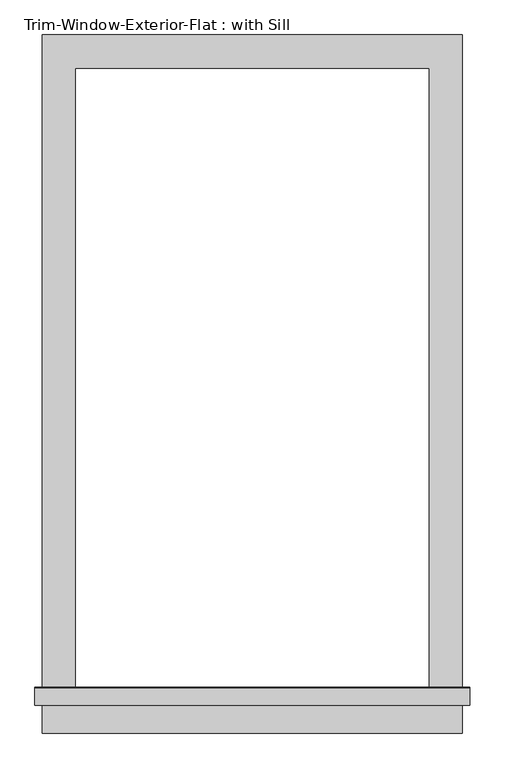
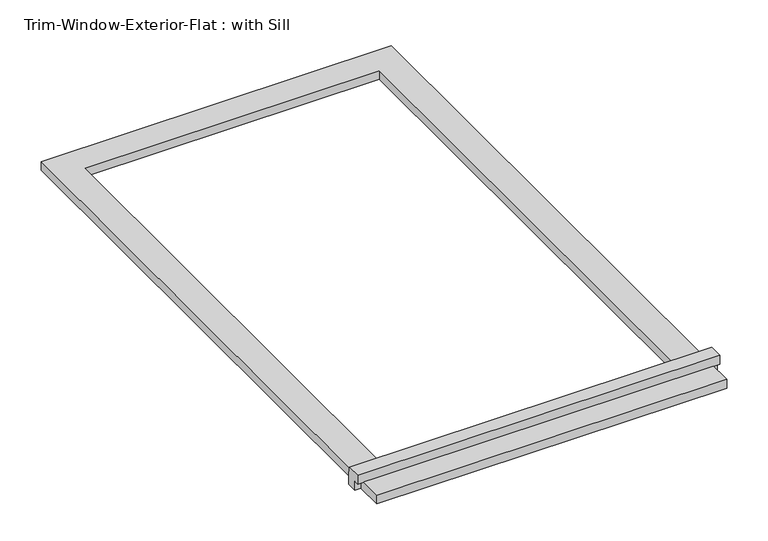
"""IFC4 building model written with IfcOpenShell, lengths in millimetres: proxy geometry, Trim-Window-Exterior-Flat : with Sill."""

from ifc_helpers import new_model, si_unit, frame, origin, origin_with_axes, place, context, project, spatial, polyline, outline, extrude, source, transform, mapped, element, save


def trim_window_exterior_flat_with_sill_278e6a94(model_context):
    return source(origin(), model_context, "Body", "SweptSolid", [
        extrude(outline(polyline([(361.95, -1088.9823709), (361.95, -1146.1323709), (-361.95, -1146.1323709), (-361.95, -1088.9823709), (361.95, -1088.9823709)])), origin_with_axes(), (0.0, 0.0, 1.0), 19.05),
        extrude(outline(polyline([(-1098.55, 38.1), (-1069.2580645, 38.1), (-1066.8, 19.05), (-1066.8, 0.0), (-1088.9823709, 0.0), (-1088.9823709, 19.05), (-1098.55, 19.05), (-1098.55, 38.1)])), frame((-374.65, 0.0, 0.0), z_axis=(1.0, 0.0, 0.0), x_axis=(0.0, 1.0, 0.0)), (0.0, 0.0, 1.0), 749.3),
        extrude(outline(polyline([(-361.95, 57.15), (361.95, 57.15), (361.95, -1066.8), (304.8, -1066.8), (304.8, 0.0), (-304.8, 0.0), (-304.8, -1066.8), (-361.95, -1066.8), (-361.95, 57.15)])), origin_with_axes(), (0.0, 0.0, 1.0), 19.05),
    ])


if __name__ == "__main__":
    model = new_model("IFC4")
    model_context = context("Model", 3, world=origin())
    ifc_project = project(units=[si_unit("LENGTHUNIT", "METRE", prefix="MILLI")], contexts=[model_context])
    site = spatial("IfcSite", under=ifc_project)
    building = spatial("IfcBuilding", under=site)
    placement = place(None, origin())
    trim_window_exterior_flat_with_sill_shape = trim_window_exterior_flat_with_sill_278e6a94(model_context)
    element("IfcBuildingElementProxy", 1, Name="Trim-Window-Exterior-Flat : with Sill", ObjectType="Trim-Window-Exterior-Flat : with Sill", at=placement, inside=building, context=model_context, shape_type="MappedRepresentation", body=[
        mapped(trim_window_exterior_flat_with_sill_shape, transform((0.0, 0.0, 0.0), x_axis=(1.0, 0.0, 0.0), y_axis=(0.0, 1.0, 0.0), z_axis=(0.0, 0.0, 1.0))),
    ])
    save(model, "model.ifc")

# Revit data of these elements
# Type "Trim-Window-Exterior-Flat : with Sill"
#   Trim Width = 0' - 2 1/4"
#   Trim Thickness_Picture Frame = 0' - 1 1/4"
#   Trim Thickness_with Sill = 0' - 0 3/4"
#   Sill Thickness = 0' - 1 1/4"
#   Opening Width [instance default] = 2' - 0"
#   Opening Height [instance default] = 3' - 0"
#   Default Elevation = 4' - 0"
#   Sill = yes
#   Picture Frame = no
#   Trim Material [instance default] = none
# Element 1 (IfcBuildingElementProxy, "Trim-Window-Exterior-Flat : with Sill")
#   Opening Height = 3' - 6"
#   Trim Material = Clad - White
#   Materials on its faces: "Clad - White"
# Materials
#   "Clad - White": class "Wood", colour RGB 242 242 238, transparency 0, Cost = 0
